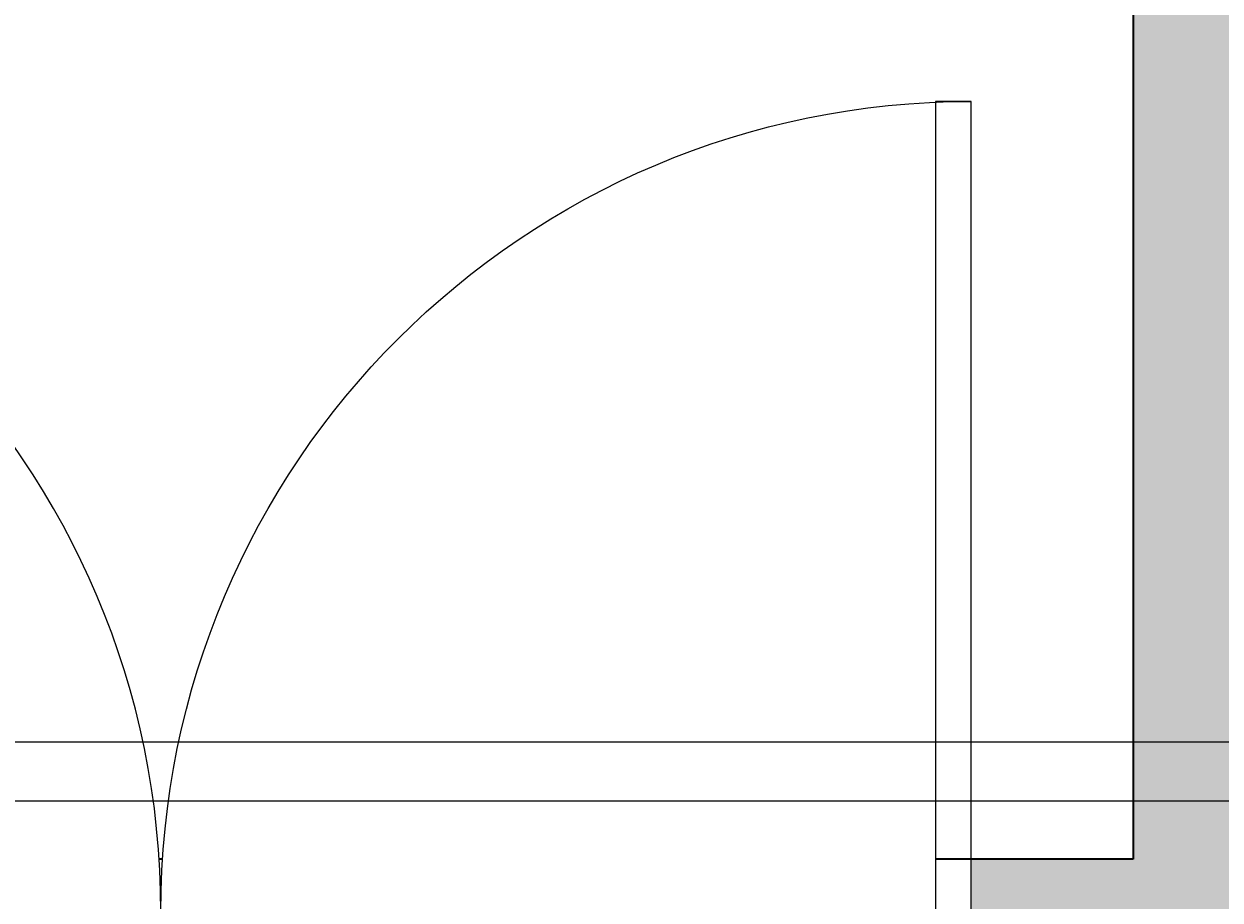
# Model space of a CAD drawing. Units: inches. Extents: x 1998 to 2588, y 1139 to 1977.
# Tile 50 of 134: x 2313 to 2344, y 1592 to 1615. Entities that reach past the tile are written whole.
import ezdxf

# ---------------------------------------------------------------- set-up
doc = ezdxf.new("R2010")
doc.units = ezdxf.units.IN
for name, color, linetype, lineweight in [('A-ANNO-DIMS', 2, 'Continuous', 18), ('A-WALL-PATT', 252, 'Continuous', 13), ('DOOR', 52, 'Continuous', 25), ('WALL', 200, 'Continuous', 35)]:
    doc.layers.add(name, color=color, linetype=linetype, lineweight=lineweight)
doc.styles.get("Standard").update_dxf_attribs({"font": 'arial.ttf'})
doc.dimstyles.get("Standard").update_dxf_attribs({"dimtxt": 0.18, "dimasz": 0.18, "dimexe": 0.18, "dimexo": 0.0625, "dimgap": 0.09, "dimtad": 0, "dimtih": 1, "dimtoh": 1, "dimdec": 4, "dimzin": 0, "dimdsep": 46, "dimtxsty": 'Standard', "dimcen": 0.09, "dimadec": 0, "dimazin": 0, "dimtfac": 1, "dimtdec": 4, "dimtofl": 0, "dimtmove": 0, "dimatfit": 3, "dimfxl": 1, "dimtolj": 1, "dimtzin": 0, "dimarcsym": 0})

# ---------------------------------------------------------------- blocks, each defined once
blk = doc.blocks.new('*U2')
for p, q in [((0, 0), (0, -6)), ((40, 0), (40, -6))]:
    blk.add_line(p, q)
blk.add_lwpolyline([(0, 0), (0, 40), (1.75, 40), (1.75, 0)], close=True)
blk.add_arc((0, 0), 40, 0, 90)
blk = doc.blocks.new('*D30')
at = {"layer": 'A-ANNO-DIMS', "color": 0, "lineweight": -2, "transparency": 16777216}
for p, q in [((2407.91, 1636.732), (1997.843, 1636.732)), ((1998.023, 1636.552), (1998.023, 1615.913)), ((1998.023, 1594.912), (1998.023, 1615.552)), ((2407.91, 1594.732), (1997.843, 1594.732))]:
    blk.add_line(p, q, dxfattribs=at)
at = {"layer": 'A-ANNO-DIMS', "color": 0, "transparency": 16777216}
for points in [[(1997.993, 1636.552), (1998.053, 1636.552), (1998.023, 1636.732)], [(1997.993, 1594.912), (1998.053, 1594.912), (1998.023, 1594.732)]]:
    blk.add_solid(points, dxfattribs=at)
at = {"layer": 'Defpoints', "color": 0, "transparency": 16777216}
for p in [(1998.023, 1636.732), (2407.973, 1636.732), (2407.973, 1594.732)]:
    blk.add_point(p, dxfattribs=at)
at = {"layer": 'A-ANNO-DIMS', "color": 0, "transparency": 16777216, "insert": (1998.023, 1615.732), "char_height": 0.18, "attachment_point": 5}
blk.add_mtext('\\A1;42', dxfattribs=at)
blk = doc.blocks.new('*D34')
at = {"layer": 'A-ANNO-DIMS', "color": 0, "lineweight": -2, "transparency": 16777216}
for p, q in [((2407.91, 1594.732), (1997.843, 1594.732)), ((1998.023, 1594.552), (1998.023, 1558.913)), ((1998.023, 1522.912), (1998.023, 1558.552)), ((2407.91, 1522.732), (1997.843, 1522.732))]:
    blk.add_line(p, q, dxfattribs=at)
at = {"layer": 'A-ANNO-DIMS', "color": 0, "transparency": 16777216}
for points in [[(1997.993, 1594.552), (1998.053, 1594.552), (1998.023, 1594.732)], [(1997.993, 1522.912), (1998.053, 1522.912), (1998.023, 1522.732)]]:
    blk.add_solid(points, dxfattribs=at)
at = {"layer": 'Defpoints', "color": 0, "transparency": 16777216}
for p in [(1998.023, 1594.732), (2407.973, 1594.732), (2407.973, 1522.732)]:
    blk.add_point(p, dxfattribs=at)
at = {"layer": 'A-ANNO-DIMS', "color": 0, "transparency": 16777216, "insert": (1998.023, 1558.732), "char_height": 0.18, "attachment_point": 5}
blk.add_mtext('\\A1;72', dxfattribs=at)
blk = doc.blocks.new('*D39')
at = {"layer": 'A-ANNO-DIMS', "color": 0, "lineweight": -2, "transparency": 16777216}
for p, q in [((2115.035, 1628.742), (2588.309, 1628.742)), ((2588.129, 1628.562), (2588.129, 1612.685)), ((2588.129, 1596.444), (2588.129, 1612.321)), ((2115.035, 1596.264), (2588.309, 1596.264))]:
    blk.add_line(p, q, dxfattribs=at)
at = {"layer": 'A-ANNO-DIMS', "color": 0, "transparency": 16777216}
for points in [[(2588.099, 1628.562), (2588.159, 1628.562), (2588.129, 1628.742)], [(2588.099, 1596.444), (2588.159, 1596.444), (2588.129, 1596.264)]]:
    blk.add_solid(points, dxfattribs=at)
at = {"layer": 'Defpoints', "color": 0, "transparency": 16777216}
for p in [(2114.973, 1628.742), (2588.129, 1628.742), (2114.973, 1596.264)]:
    blk.add_point(p, dxfattribs=at)
at = {"layer": 'A-ANNO-DIMS', "color": 0, "transparency": 16777216, "insert": (2588.129, 1612.503), "char_height": 0.18, "attachment_point": 5}
blk.add_mtext('\\A1;32.48', dxfattribs=at)

msp = doc.modelspace()

# ---------------------------------------------------------------- hatches: boundary and pattern name
at = {"layer": 'A-WALL-PATT'}
h = msp.add_hatch(color=256, dxfattribs=at)
h.dxf.hatch_style = 1
h.paths.add_polyline_path([(2222.9729, 1888.7324), (2099.4125, 1888.7324), (2099.4125, 1879.7324), (2222.9729, 1879.7324)])
h.paths.add_polyline_path([(2096.9729, 1868.3278), (2087.9729, 1868.3278), (2087.9729, 1775.637), (2096.9729, 1775.637)])
h.paths.add_polyline_path([(2227.4729, 1868.3278), (2222.9729, 1868.3278), (2222.9729, 1774.3318), (2227.4729, 1774.3318)])
h.paths.add_polyline_path([(2188.3019, 1759.7324), (2138.6074, 1759.7324), (2099.4125, 1759.7324), (2099.4125, 1755.2324), (2176.9729, 1755.2324), (2188.3019, 1755.2324)])
h.paths.add_polyline_path([(2087.9729, 1759.7324), (2059.4729, 1759.7324), (2059.4729, 1702.7324), (2087.9729, 1702.7324), (2087.9729, 1707.2324), (2063.9729, 1707.2324), (2063.9729, 1755.2324), (2087.9729, 1755.2324)])
h.paths.add_polyline_path([(2096.9729, 1755.2324), (2087.9729, 1755.2324), (2087.9729, 1707.2324), (2096.9729, 1707.2324)])
h.paths.add_polyline_path([(2187.0461, 1707.2324), (2105.9729, 1707.2324), (2096.9729, 1707.2324), (2087.9729, 1707.2324), (2087.9729, 1702.7324), (2105.9729, 1702.7324), (2114.9729, 1702.7324), (2187.0461, 1702.7324)])
h.paths.add_polyline_path([(2181.4729, 1719.2028), (2176.9729, 1719.2028), (2176.9729, 1707.2324), (2181.4729, 1707.2324)])
h.paths.add_polyline_path([(2216.0332, 1588.7324), (2114.9729, 1588.7324), (2105.9729, 1588.7324), (2105.9729, 1584.2324), (2216.0332, 1584.2324)])
h.paths.add_polyline_path([(2077.691, 1588.7324), (2061.4729, 1588.7324), (2061.4729, 1584.2324), (2077.691, 1584.2324)])
h.paths.add_polyline_path([(2105.9729, 1588.7324), (2098.0956, 1588.7324), (2098.0956, 1584.2324), (2105.9729, 1584.2324)])
h.paths.add_polyline_path([(2114.9729, 1596.2642), (2110.1012, 1596.2642), (2105.9729, 1596.2642), (2105.9729, 1588.7324), (2114.9729, 1588.7324)])
h.paths.add_polyline_path([(2114.9729, 1584.2324), (2105.9729, 1584.2324), (2105.9729, 1580.249), (2110.1012, 1580.249), (2114.9729, 1580.249)])
h.paths.add_polyline_path([(2114.9729, 1547.7716), (2110.1012, 1547.7716, -0.0318759), (2105.9729, 1548.035), (2105.9729, 1470.2324), (2108.3775, 1470.2324), (2108.3775, 1465.7324), (2186.2943, 1465.7324), (2186.2943, 1470.2324), (2114.9729, 1470.2324)])
h.paths.add_polyline_path([(2227.4729, 1584.2324), (2222.9729, 1584.2324), (2222.9729, 1486.137), (2227.4729, 1486.137)])
h.paths.add_polyline_path([(2295.4138, 1593.2324), (2227.4729, 1593.2324), (2227.4729, 1588.7324), (2295.4138, 1588.7324), (2295.4138, 1591.8729)])
h.paths.add_polyline_path([(2345.9729, 1627.1165), (2341.4729, 1627.1165), (2341.4729, 1593.2324), (2337.2869, 1593.2324), (2337.2869, 1591.8729), (2337.2869, 1588.7324), (2345.9729, 1588.7324)])
h.paths.add_polyline_path([(2291.9729, 1588.7324), (2287.4729, 1588.7324), (2287.4729, 1522.7324), (2291.9729, 1522.7324)])
h.paths.add_polyline_path([(2291.9729, 1522.7324), (2287.4729, 1522.7324), (2227.4729, 1522.7324), (2227.4729, 1518.2324), (2291.9729, 1518.2324)])
h.paths.add_polyline_path([(2295.7347, 1519.5919), (2295.7347, 1522.7324), (2291.9729, 1522.7324), (2291.9729, 1518.2324), (2295.7347, 1518.2324)])
h.paths.add_polyline_path([(2345.9729, 1522.7324), (2337.6078, 1522.7324), (2337.6078, 1519.5919), (2337.6078, 1518.2324), (2341.4729, 1518.2324), (2341.4729, 1488.5616), (2345.9729, 1488.5616)])
h.paths.add_polyline_path([(2345.9729, 1468.1569), (2341.4729, 1468.1569), (2341.4729, 1374.2324), (2227.4729, 1374.2324), (2227.4729, 1369.7324), (2345.9729, 1369.7324)])
h.paths.add_polyline_path([(2345.9729, 1369.7324), (2341.4729, 1369.7324), (2341.4729, 1362.2324), (2345.9729, 1362.2324)])
h.paths.add_polyline_path([(2345.9729, 1317.7324), (2345.9729, 1322.2324), (2341.4729, 1322.2324), (2341.4729, 1285.137), (2345.9729, 1285.137)], flags=17)
h.paths.add_polyline_path([(2356.2096, 1322.2324), (2345.9729, 1322.2324), (2345.9729, 1317.7324), (2356.2096, 1317.7324), (2356.2096, 1319.3088)], flags=17)
h.paths.add_polyline_path([(2393.9729, 1322.2324), (2375.6999, 1322.2324), (2375.6999, 1319.3088, -0.0202458), (2375.636, 1317.7324), (2393.9729, 1317.7324)], flags=17)
h.paths.add_polyline_path([(2398.4729, 1322.2324), (2393.9729, 1322.2324), (2393.9729, 1317.7324), (2393.9729, 1237.7324), (2345.9729, 1237.7324), (2345.9729, 1264.7324), (2341.4729, 1264.7324), (2341.4729, 1228.7324), (2393.9729, 1228.7324), (2482.7412, 1228.7324), (2482.7412, 1237.7324), (2398.4729, 1237.7324), (2398.4729, 1297.1029)])
h.paths.add_polyline_path([(2398.4729, 1362.2324), (2393.9729, 1362.2324), (2393.9729, 1357.7324), (2398.4729, 1357.7324)])
h.paths.add_polyline_path([(2345.9729, 1329.7549), (2341.4729, 1329.7549), (2341.4729, 1322.2324), (2345.9729, 1322.2324)])

# ---------------------------------------------------------------- linework, layer by layer
at = {"layer": 'WALL'}
for p, q in [((2341.4729, 1627.1165), (2341.4729, 1593.2324)), ((2316.3945, 1593.2324), (2316.3062, 1593.2324)), ((2341.4729, 1593.2324), (2336.3709, 1593.2324))]:
    msp.add_line(p, q, dxfattribs=at)

# ---------------------------------------------------------------- block references
at = {"layer": 'DOOR', "yscale": 0.5234138920659225, "zscale": 0.5234138920659225}
for p, xscale in [((2295.4138, 1591.8729), 0.5234138920659225), ((2337.2869, 1591.8729), -0.5234138920659225)]:
    msp.add_blockref('*U2', p, dxfattribs=dict(at, xscale=xscale))

# ---------------------------------------------------------------- dimensions: what is measured, and where the dimension line sits
at = {"layer": 'A-ANNO-DIMS'}
for base, p1, p2, override, picture, middle in [((1998.0229, 1636.7324), (2407.9729, 1594.7324), (2407.9729, 1636.7324), {"dimdec": 0, "dimlfac": 1, "dimrnd": 0, "dimzin": 0, "dimdsep": 46, "dimlunit": 2}, '*D30', (1998.0229, 1615.7324)), ((2588.1286, 1628.7416), (2114.9729, 1596.2642), (2114.9729, 1628.7416), {"dimdec": 2, "dimlfac": 1, "dimrnd": 0, "dimzin": 0, "dimdsep": 46, "dimlunit": 2}, '*D39', (2588.1286, 1612.5029)), ((1998.0229, 1594.7324), (2407.9729, 1522.7324), (2407.9729, 1594.7324), {"dimdec": 0, "dimlfac": 1, "dimrnd": 0, "dimzin": 0, "dimdsep": 46, "dimlunit": 2}, '*D34', (1998.0229, 1558.7324))]:
    dim = msp.add_linear_dim(base=base, p1=p1, p2=p2, angle=90, dimstyle='Standard', override=override, dxfattribs=at)
    dim.commit()
    dim.dimension.update_dxf_attribs({"geometry": picture, "text_midpoint": middle})

doc.saveas('drawing.dxf')
